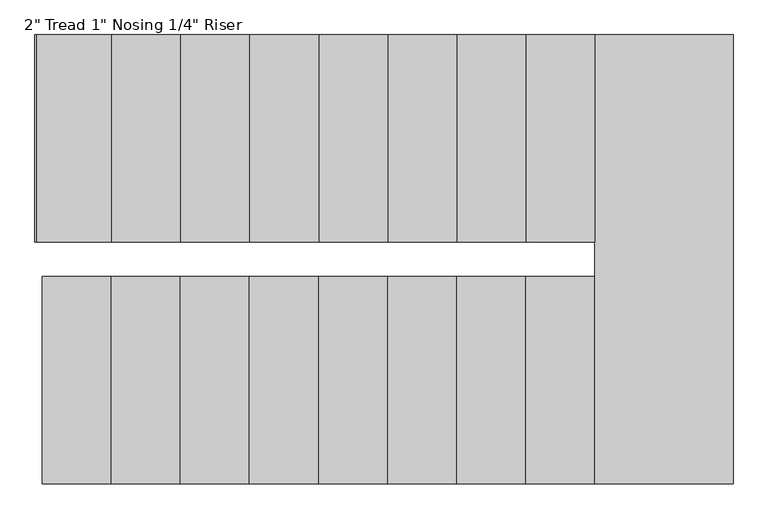
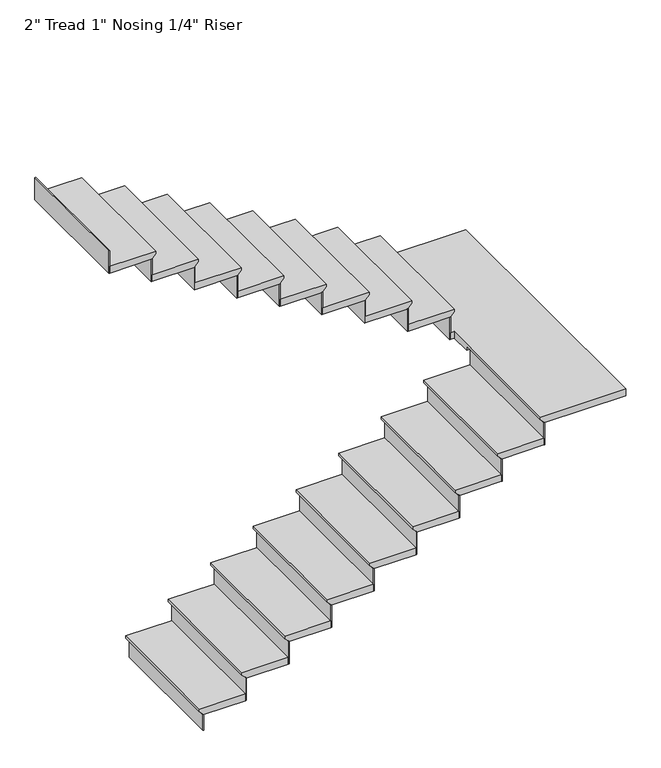
"""IFC4 building model written with IfcOpenShell, lengths in millimetres: stair flight geometry."""

from ifc_helpers import new_model, si_unit, origin, place, context, project, spatial, faceted_brep, source, transform, mapped, element, save


def stair_flight_21a7b5a9(model_context):
    return source(origin(), model_context, "Body", "Brep", [
        faceted_brep([(-1197.97188, -4816.50869, 3198.2833333), (-1197.97188, -4816.50869, 3217.3333333), (-1197.97188, -3902.10869, 3217.3333333), (-1197.97188, -3902.10869, 3198.2833333), (-1172.57188, -4816.50869, 3172.8833333), (-1172.57188, -3902.10869, 3172.8833333), (-867.77188, -4816.50869, 3217.3333333), (-867.77188, -3902.10869, 3217.3333333), (-1172.57188, -3902.10869, 3166.5333333), (-867.77188, -3902.10869, 3166.5333333), (-867.77188, -4816.50869, 3166.5333333), (-1172.57188, -4816.50869, 3166.5333333)], [[[0, 1, 2, 3]], [[4, 0, 3, 5]], [[2, 1, 6, 7]], [[8, 9, 10, 11]], [[2, 7, 9, 8, 5, 3]], [[8, 11, 4, 5]], [[6, 1, 0, 4, 11, 10]], [[7, 6, 10, 9]]]),
        faceted_brep([(-1172.57188, -4816.50869, 3166.5333333), (-1172.57188, -4816.50869, 3048.0), (-1166.22188, -4816.50869, 3048.0), (-1166.22188, -4816.50869, 3166.5333333), (-1172.57188, -3902.10869, 3166.5333333), (-1166.22188, -3902.10869, 3166.5333333), (-1166.22188, -3902.10869, 3048.0), (-1172.57188, -3902.10869, 3048.0)], [[[0, 1, 2, 3]], [[4, 5, 6, 7]], [[1, 0, 4, 7]], [[2, 1, 7, 6]], [[3, 2, 6, 5]], [[0, 3, 5, 4]]]),
        faceted_brep([(-867.77188, -4816.50869, 3335.8666667), (-867.77188, -4816.50869, 3166.5333333), (-861.42188, -4816.50869, 3166.5333333), (-861.42188, -4816.50869, 3335.8666667), (-867.77188, -3902.10869, 3335.8666667), (-861.42188, -3902.10869, 3335.8666667), (-861.42188, -3902.10869, 3166.5333333), (-867.77188, -3902.10869, 3166.5333333)], [[[0, 1, 2, 3]], [[4, 5, 6, 7]], [[1, 0, 4, 7]], [[2, 1, 7, 6]], [[3, 2, 6, 5]], [[0, 3, 5, 4]]]),
        faceted_brep([(-893.17188, -3902.10869, 3386.6666667), (-893.17188, -4816.50869, 3386.6666667), (-562.97188, -4816.50869, 3386.6666667), (-562.97188, -3902.10869, 3386.6666667), (-867.77188, -3902.10869, 3335.8666667), (-562.97188, -3902.10869, 3335.8666667), (-562.97188, -4816.50869, 3335.8666667), (-867.77188, -4816.50869, 3335.8666667), (-867.77188, -3902.10869, 3342.2166667), (-893.17188, -3902.10869, 3367.6166667), (-867.77188, -4816.50869, 3342.2166667), (-893.17188, -4816.50869, 3367.6166667)], [[[0, 1, 2, 3]], [[4, 5, 6, 7]], [[0, 3, 5, 4, 8, 9]], [[4, 7, 10, 8]], [[2, 1, 11, 10, 7, 6]], [[3, 2, 6, 5]], [[11, 1, 0, 9]], [[10, 11, 9, 8]]]),
        faceted_brep([(-562.97188, -4816.50869, 3505.2), (-562.97188, -4816.50869, 3335.8666667), (-556.62188, -4816.50869, 3335.8666667), (-556.62188, -4816.50869, 3505.2), (-562.97188, -3902.10869, 3505.2), (-556.62188, -3902.10869, 3505.2), (-556.62188, -3902.10869, 3335.8666667), (-562.97188, -3902.10869, 3335.8666667)], [[[0, 1, 2, 3]], [[4, 5, 6, 7]], [[1, 0, 4, 7]], [[2, 1, 7, 6]], [[3, 2, 6, 5]], [[0, 3, 5, 4]]]),
        faceted_brep([(-588.37188, -3902.10869, 3556.0), (-588.37188, -4816.50869, 3556.0), (-258.17188, -4816.50869, 3556.0), (-258.17188, -3902.10869, 3556.0), (-562.97188, -3902.10869, 3505.2), (-258.17188, -3902.10869, 3505.2), (-258.17188, -4816.50869, 3505.2), (-562.97188, -4816.50869, 3505.2), (-562.97188, -3902.10869, 3511.55), (-588.37188, -3902.10869, 3536.95), (-562.97188, -4816.50869, 3511.55), (-588.37188, -4816.50869, 3536.95)], [[[0, 1, 2, 3]], [[4, 5, 6, 7]], [[0, 3, 5, 4, 8, 9]], [[4, 7, 10, 8]], [[2, 1, 11, 10, 7, 6]], [[3, 2, 6, 5]], [[11, 1, 0, 9]], [[10, 11, 9, 8]]]),
        faceted_brep([(-258.17188, -4816.50869, 3674.5333333), (-258.17188, -4816.50869, 3505.2), (-251.82188, -4816.50869, 3505.2), (-251.82188, -4816.50869, 3674.5333333), (-258.17188, -3902.10869, 3674.5333333), (-251.82188, -3902.10869, 3674.5333333), (-251.82188, -3902.10869, 3505.2), (-258.17188, -3902.10869, 3505.2)], [[[0, 1, 2, 3]], [[4, 5, 6, 7]], [[1, 0, 4, 7]], [[2, 1, 7, 6]], [[3, 2, 6, 5]], [[0, 3, 5, 4]]]),
        faceted_brep([(-283.57188, -3902.10869, 3725.3333333), (-283.57188, -4816.50869, 3725.3333333), (46.62812, -4816.50869, 3725.3333333), (46.62812, -3902.10869, 3725.3333333), (-258.17188, -3902.10869, 3674.5333333), (46.62812, -3902.10869, 3674.5333333), (46.62812, -4816.50869, 3674.5333333), (-258.17188, -4816.50869, 3674.5333333), (-258.17188, -3902.10869, 3680.8833333), (-283.57188, -3902.10869, 3706.2833333), (-258.17188, -4816.50869, 3680.8833333), (-283.57188, -4816.50869, 3706.2833333)], [[[0, 1, 2, 3]], [[4, 5, 6, 7]], [[0, 3, 5, 4, 8, 9]], [[4, 7, 10, 8]], [[2, 1, 11, 10, 7, 6]], [[3, 2, 6, 5]], [[11, 1, 0, 9]], [[10, 11, 9, 8]]]),
        faceted_brep([(46.62812, -4816.50869, 3843.8666667), (46.62812, -4816.50869, 3674.5333333), (52.97812, -4816.50869, 3674.5333333), (52.97812, -4816.50869, 3843.8666667), (46.62812, -3902.10869, 3843.8666667), (52.97812, -3902.10869, 3843.8666667), (52.97812, -3902.10869, 3674.5333333), (46.62812, -3902.10869, 3674.5333333)], [[[0, 1, 2, 3]], [[4, 5, 6, 7]], [[1, 0, 4, 7]], [[2, 1, 7, 6]], [[3, 2, 6, 5]], [[0, 3, 5, 4]]]),
        faceted_brep([(21.22812, -3902.10869, 3894.6666667), (21.22812, -4816.50869, 3894.6666667), (351.42812, -4816.50869, 3894.6666667), (351.42812, -3902.10869, 3894.6666667), (46.62812, -3902.10869, 3843.8666667), (351.42812, -3902.10869, 3843.8666667), (351.42812, -4816.50869, 3843.8666667), (46.62812, -4816.50869, 3843.8666667), (46.62812, -3902.10869, 3850.2166667), (21.22812, -3902.10869, 3875.6166667), (46.62812, -4816.50869, 3850.2166667), (21.22812, -4816.50869, 3875.6166667)], [[[0, 1, 2, 3]], [[4, 5, 6, 7]], [[0, 3, 5, 4, 8, 9]], [[4, 7, 10, 8]], [[2, 1, 11, 10, 7, 6]], [[3, 2, 6, 5]], [[11, 1, 0, 9]], [[10, 11, 9, 8]]]),
        faceted_brep([(351.42812, -4816.50869, 4013.2), (351.42812, -4816.50869, 3843.8666667), (357.77812, -4816.50869, 3843.8666667), (357.77812, -4816.50869, 4013.2), (351.42812, -3902.10869, 4013.2), (357.77812, -3902.10869, 4013.2), (357.77812, -3902.10869, 3843.8666667), (351.42812, -3902.10869, 3843.8666667)], [[[0, 1, 2, 3]], [[4, 5, 6, 7]], [[1, 0, 4, 7]], [[2, 1, 7, 6]], [[3, 2, 6, 5]], [[0, 3, 5, 4]]]),
        faceted_brep([(326.02812, -3902.10869, 4064.0), (326.02812, -4816.50869, 4064.0), (656.22812, -4816.50869, 4064.0), (656.22812, -3902.10869, 4064.0), (351.42812, -3902.10869, 4013.2), (656.22812, -3902.10869, 4013.2), (656.22812, -4816.50869, 4013.2), (351.42812, -4816.50869, 4013.2), (351.42812, -3902.10869, 4019.55), (326.02812, -3902.10869, 4044.95), (351.42812, -4816.50869, 4019.55), (326.02812, -4816.50869, 4044.95)], [[[0, 1, 2, 3]], [[4, 5, 6, 7]], [[0, 3, 5, 4, 8, 9]], [[4, 7, 10, 8]], [[2, 1, 11, 10, 7, 6]], [[3, 2, 6, 5]], [[11, 1, 0, 9]], [[10, 11, 9, 8]]]),
        faceted_brep([(656.22812, -4816.50869, 4182.5333333), (656.22812, -4816.50869, 4013.2), (662.57812, -4816.50869, 4013.2), (662.57812, -4816.50869, 4182.5333333), (656.22812, -3902.10869, 4182.5333333), (662.57812, -3902.10869, 4182.5333333), (662.57812, -3902.10869, 4013.2), (656.22812, -3902.10869, 4013.2)], [[[0, 1, 2, 3]], [[4, 5, 6, 7]], [[1, 0, 4, 7]], [[2, 1, 7, 6]], [[3, 2, 6, 5]], [[0, 3, 5, 4]]]),
        faceted_brep([(630.82812, -3902.10869, 4233.3333333), (630.82812, -4816.50869, 4233.3333333), (961.02812, -4816.50869, 4233.3333333), (961.02812, -3902.10869, 4233.3333333), (656.22812, -3902.10869, 4182.5333333), (961.02812, -3902.10869, 4182.5333333), (961.02812, -4816.50869, 4182.5333333), (656.22812, -4816.50869, 4182.5333333), (656.22812, -3902.10869, 4188.8833333), (630.82812, -3902.10869, 4214.2833333), (656.22812, -4816.50869, 4188.8833333), (630.82812, -4816.50869, 4214.2833333)], [[[0, 1, 2, 3]], [[4, 5, 6, 7]], [[0, 3, 5, 4, 8, 9]], [[4, 7, 10, 8]], [[2, 1, 11, 10, 7, 6]], [[3, 2, 6, 5]], [[11, 1, 0, 9]], [[10, 11, 9, 8]]]),
        faceted_brep([(961.02812, -4816.50869, 4351.8666667), (961.02812, -4816.50869, 4182.5333333), (967.37812, -4816.50869, 4182.5333333), (967.37812, -4816.50869, 4351.8666667), (961.02812, -3902.10869, 4351.8666667), (967.37812, -3902.10869, 4351.8666667), (967.37812, -3902.10869, 4182.5333333), (961.02812, -3902.10869, 4182.5333333)], [[[0, 1, 2, 3]], [[4, 5, 6, 7]], [[1, 0, 4, 7]], [[2, 1, 7, 6]], [[3, 2, 6, 5]], [[0, 3, 5, 4]]]),
        faceted_brep([(935.62812, -3902.10869, 4402.6666667), (935.62812, -4816.50869, 4402.6666667), (1265.82812, -4816.50869, 4402.6666667), (1265.82812, -3902.10869, 4402.6666667), (961.02812, -3902.10869, 4351.8666667), (1265.82812, -3902.10869, 4351.8666667), (1265.82812, -4816.50869, 4351.8666667), (961.02812, -4816.50869, 4351.8666667), (961.02812, -3902.10869, 4358.2166667), (935.62812, -3902.10869, 4383.6166667), (961.02812, -4816.50869, 4358.2166667), (935.62812, -4816.50869, 4383.6166667)], [[[0, 1, 2, 3]], [[4, 5, 6, 7]], [[0, 3, 5, 4, 8, 9]], [[4, 7, 10, 8]], [[2, 1, 11, 10, 7, 6]], [[3, 2, 6, 5]], [[11, 1, 0, 9]], [[10, 11, 9, 8]]]),
        faceted_brep([(1265.82812, -4816.50869, 4521.2), (1265.82812, -4816.50869, 4351.8666667), (1272.17812, -4816.50869, 4351.8666667), (1272.17812, -4816.50869, 4521.2), (1265.82812, -3902.10869, 4521.2), (1272.17812, -3902.10869, 4521.2), (1272.17812, -3902.10869, 4351.8666667), (1265.82812, -3902.10869, 4351.8666667)], [[[0, 1, 2, 3]], [[4, 5, 6, 7]], [[1, 0, 4, 7]], [[2, 1, 7, 6]], [[3, 2, 6, 5]], [[0, 3, 5, 4]]]),
        faceted_brep([(1215.02812, -3749.70869, 4572.0), (1240.42812, -3749.70869, 4572.0), (1240.42812, -4816.50869, 4572.0), (1850.02812, -4816.50869, 4572.0), (1850.02812, -2835.30869, 4572.0), (1215.02812, -2835.30869, 4572.0), (1240.42812, -3749.70869, 4521.2), (1215.02812, -3749.70869, 4521.2), (1215.02812, -2835.30869, 4521.2), (1850.02812, -2835.30869, 4521.2), (1850.02812, -4816.50869, 4521.2), (1265.82812, -4816.50869, 4521.2), (1265.82812, -3902.10869, 4521.2), (1240.42812, -3902.10869, 4521.2), (1240.42812, -3902.10869, 4552.95), (1240.42812, -4816.50869, 4552.95), (1265.82812, -3902.10869, 4527.55), (1265.82812, -4816.50869, 4527.55)], [[[0, 1, 2, 3, 4, 5]], [[6, 7, 8, 9, 10, 11, 12, 13]], [[1, 0, 7, 6]], [[2, 1, 6, 13, 14, 15]], [[13, 12, 16, 14]], [[12, 11, 17, 16]], [[3, 2, 15, 17, 11, 10]], [[4, 3, 10, 9]], [[5, 4, 9, 8]], [[0, 5, 8, 7]], [[17, 15, 14, 16]]]),
        faceted_brep([(1215.02812, -2835.30869, 4690.5333333), (1215.02812, -2835.30869, 4521.2), (1208.67812, -2835.30869, 4521.2), (1208.67812, -2835.30869, 4690.5333333), (1215.02812, -3749.70869, 4690.5333333), (1208.67812, -3749.70869, 4690.5333333), (1208.67812, -3749.70869, 4521.2), (1215.02812, -3749.70869, 4521.2)], [[[0, 1, 2, 3]], [[4, 5, 6, 7]], [[1, 0, 4, 7]], [[2, 1, 7, 6]], [[3, 2, 6, 5]], [[0, 3, 5, 4]]]),
        faceted_brep([(1240.42812, -3749.70869, 4741.3333333), (1240.42812, -2835.30869, 4741.3333333), (910.22812, -2835.30869, 4741.3333333), (910.22812, -3749.70869, 4741.3333333), (1215.02812, -3749.70869, 4690.5333333), (910.22812, -3749.70869, 4690.5333333), (910.22812, -2835.30869, 4690.5333333), (1215.02812, -2835.30869, 4690.5333333), (1215.02812, -3749.70869, 4696.8833333), (1240.42812, -3749.70869, 4722.2833333), (1215.02812, -2835.30869, 4696.8833333), (1240.42812, -2835.30869, 4722.2833333)], [[[0, 1, 2, 3]], [[4, 5, 6, 7]], [[0, 3, 5, 4, 8, 9]], [[4, 7, 10, 8]], [[2, 1, 11, 10, 7, 6]], [[3, 2, 6, 5]], [[11, 1, 0, 9]], [[10, 11, 9, 8]]]),
        faceted_brep([(910.22812, -2835.30869, 4859.8666667), (910.22812, -2835.30869, 4690.5333333), (903.87812, -2835.30869, 4690.5333333), (903.87812, -2835.30869, 4859.8666667), (910.22812, -3749.70869, 4859.8666667), (903.87812, -3749.70869, 4859.8666667), (903.87812, -3749.70869, 4690.5333333), (910.22812, -3749.70869, 4690.5333333)], [[[0, 1, 2, 3]], [[4, 5, 6, 7]], [[1, 0, 4, 7]], [[2, 1, 7, 6]], [[3, 2, 6, 5]], [[0, 3, 5, 4]]]),
        faceted_brep([(935.62812, -3749.70869, 4910.6666667), (935.62812, -2835.30869, 4910.6666667), (605.42812, -2835.30869, 4910.6666667), (605.42812, -3749.70869, 4910.6666667), (910.22812, -3749.70869, 4859.8666667), (605.42812, -3749.70869, 4859.8666667), (605.42812, -2835.30869, 4859.8666667), (910.22812, -2835.30869, 4859.8666667), (910.22812, -3749.70869, 4866.2166667), (935.62812, -3749.70869, 4891.6166667), (910.22812, -2835.30869, 4866.2166667), (935.62812, -2835.30869, 4891.6166667)], [[[0, 1, 2, 3]], [[4, 5, 6, 7]], [[0, 3, 5, 4, 8, 9]], [[4, 7, 10, 8]], [[2, 1, 11, 10, 7, 6]], [[3, 2, 6, 5]], [[11, 1, 0, 9]], [[10, 11, 9, 8]]]),
        faceted_brep([(605.42812, -2835.30869, 5029.2), (605.42812, -2835.30869, 4859.8666667), (599.07812, -2835.30869, 4859.8666667), (599.07812, -2835.30869, 5029.2), (605.42812, -3749.70869, 5029.2), (599.07812, -3749.70869, 5029.2), (599.07812, -3749.70869, 4859.8666667), (605.42812, -3749.70869, 4859.8666667)], [[[0, 1, 2, 3]], [[4, 5, 6, 7]], [[1, 0, 4, 7]], [[2, 1, 7, 6]], [[3, 2, 6, 5]], [[0, 3, 5, 4]]]),
        faceted_brep([(630.82812, -3749.70869, 5080.0), (630.82812, -2835.30869, 5080.0), (300.62812, -2835.30869, 5080.0), (300.62812, -3749.70869, 5080.0), (605.42812, -3749.70869, 5029.2), (300.62812, -3749.70869, 5029.2), (300.62812, -2835.30869, 5029.2), (605.42812, -2835.30869, 5029.2), (605.42812, -3749.70869, 5035.55), (630.82812, -3749.70869, 5060.95), (605.42812, -2835.30869, 5035.55), (630.82812, -2835.30869, 5060.95)], [[[0, 1, 2, 3]], [[4, 5, 6, 7]], [[0, 3, 5, 4, 8, 9]], [[4, 7, 10, 8]], [[2, 1, 11, 10, 7, 6]], [[3, 2, 6, 5]], [[11, 1, 0, 9]], [[10, 11, 9, 8]]]),
        faceted_brep([(300.62812, -2835.30869, 5198.5333333), (300.62812, -2835.30869, 5029.2), (294.27812, -2835.30869, 5029.2), (294.27812, -2835.30869, 5198.5333333), (300.62812, -3749.70869, 5198.5333333), (294.27812, -3749.70869, 5198.5333333), (294.27812, -3749.70869, 5029.2), (300.62812, -3749.70869, 5029.2)], [[[0, 1, 2, 3]], [[4, 5, 6, 7]], [[1, 0, 4, 7]], [[2, 1, 7, 6]], [[3, 2, 6, 5]], [[0, 3, 5, 4]]]),
        faceted_brep([(326.02812, -3749.70869, 5249.3333333), (326.02812, -2835.30869, 5249.3333333), (-4.17188, -2835.30869, 5249.3333333), (-4.17188, -3749.70869, 5249.3333333), (300.62812, -3749.70869, 5198.5333333), (-4.17188, -3749.70869, 5198.5333333), (-4.17188, -2835.30869, 5198.5333333), (300.62812, -2835.30869, 5198.5333333), (300.62812, -3749.70869, 5204.8833333), (326.02812, -3749.70869, 5230.2833333), (300.62812, -2835.30869, 5204.8833333), (326.02812, -2835.30869, 5230.2833333)], [[[0, 1, 2, 3]], [[4, 5, 6, 7]], [[0, 3, 5, 4, 8, 9]], [[4, 7, 10, 8]], [[2, 1, 11, 10, 7, 6]], [[3, 2, 6, 5]], [[11, 1, 0, 9]], [[10, 11, 9, 8]]]),
        faceted_brep([(-4.17188, -2835.30869, 5367.8666667), (-4.17188, -2835.30869, 5198.5333333), (-10.52188, -2835.30869, 5198.5333333), (-10.52188, -2835.30869, 5367.8666667), (-4.17188, -3749.70869, 5367.8666667), (-10.52188, -3749.70869, 5367.8666667), (-10.52188, -3749.70869, 5198.5333333), (-4.17188, -3749.70869, 5198.5333333)], [[[0, 1, 2, 3]], [[4, 5, 6, 7]], [[1, 0, 4, 7]], [[2, 1, 7, 6]], [[3, 2, 6, 5]], [[0, 3, 5, 4]]]),
        faceted_brep([(21.22812, -3749.70869, 5418.6666667), (21.22812, -2835.30869, 5418.6666667), (-308.97188, -2835.30869, 5418.6666667), (-308.97188, -3749.70869, 5418.6666667), (-4.17188, -3749.70869, 5367.8666667), (-308.97188, -3749.70869, 5367.8666667), (-308.97188, -2835.30869, 5367.8666667), (-4.17188, -2835.30869, 5367.8666667), (-4.17188, -3749.70869, 5374.2166667), (21.22812, -3749.70869, 5399.6166667), (-4.17188, -2835.30869, 5374.2166667), (21.22812, -2835.30869, 5399.6166667)], [[[0, 1, 2, 3]], [[4, 5, 6, 7]], [[0, 3, 5, 4, 8, 9]], [[4, 7, 10, 8]], [[2, 1, 11, 10, 7, 6]], [[3, 2, 6, 5]], [[11, 1, 0, 9]], [[10, 11, 9, 8]]]),
        faceted_brep([(-308.97188, -2835.30869, 5537.2), (-308.97188, -2835.30869, 5367.8666667), (-315.32188, -2835.30869, 5367.8666667), (-315.32188, -2835.30869, 5537.2), (-308.97188, -3749.70869, 5537.2), (-315.32188, -3749.70869, 5537.2), (-315.32188, -3749.70869, 5367.8666667), (-308.97188, -3749.70869, 5367.8666667)], [[[0, 1, 2, 3]], [[4, 5, 6, 7]], [[1, 0, 4, 7]], [[2, 1, 7, 6]], [[3, 2, 6, 5]], [[0, 3, 5, 4]]]),
        faceted_brep([(-283.57188, -3749.70869, 5588.0), (-283.57188, -2835.30869, 5588.0), (-613.77188, -2835.30869, 5588.0), (-613.77188, -3749.70869, 5588.0), (-308.97188, -3749.70869, 5537.2), (-613.77188, -3749.70869, 5537.2), (-613.77188, -2835.30869, 5537.2), (-308.97188, -2835.30869, 5537.2), (-308.97188, -3749.70869, 5543.55), (-283.57188, -3749.70869, 5568.95), (-308.97188, -2835.30869, 5543.55), (-283.57188, -2835.30869, 5568.95)], [[[0, 1, 2, 3]], [[4, 5, 6, 7]], [[0, 3, 5, 4, 8, 9]], [[4, 7, 10, 8]], [[2, 1, 11, 10, 7, 6]], [[3, 2, 6, 5]], [[11, 1, 0, 9]], [[10, 11, 9, 8]]]),
        faceted_brep([(-613.77188, -2835.30869, 5706.5333333), (-613.77188, -2835.30869, 5537.2), (-620.12188, -2835.30869, 5537.2), (-620.12188, -2835.30869, 5706.5333333), (-613.77188, -3749.70869, 5706.5333333), (-620.12188, -3749.70869, 5706.5333333), (-620.12188, -3749.70869, 5537.2), (-613.77188, -3749.70869, 5537.2)], [[[0, 1, 2, 3]], [[4, 5, 6, 7]], [[1, 0, 4, 7]], [[2, 1, 7, 6]], [[3, 2, 6, 5]], [[0, 3, 5, 4]]]),
        faceted_brep([(-588.37188, -3749.70869, 5757.3333333), (-588.37188, -2835.30869, 5757.3333333), (-918.57188, -2835.30869, 5757.3333333), (-918.57188, -3749.70869, 5757.3333333), (-613.77188, -3749.70869, 5706.5333333), (-918.57188, -3749.70869, 5706.5333333), (-918.57188, -2835.30869, 5706.5333333), (-613.77188, -2835.30869, 5706.5333333), (-613.77188, -3749.70869, 5712.8833333), (-588.37188, -3749.70869, 5738.2833333), (-613.77188, -2835.30869, 5712.8833333), (-588.37188, -2835.30869, 5738.2833333)], [[[0, 1, 2, 3]], [[4, 5, 6, 7]], [[0, 3, 5, 4, 8, 9]], [[4, 7, 10, 8]], [[2, 1, 11, 10, 7, 6]], [[3, 2, 6, 5]], [[11, 1, 0, 9]], [[10, 11, 9, 8]]]),
        faceted_brep([(-918.57188, -2835.30869, 5875.8666667), (-918.57188, -2835.30869, 5706.5333333), (-924.92188, -2835.30869, 5706.5333333), (-924.92188, -2835.30869, 5875.8666667), (-918.57188, -3749.70869, 5875.8666667), (-924.92188, -3749.70869, 5875.8666667), (-924.92188, -3749.70869, 5706.5333333), (-918.57188, -3749.70869, 5706.5333333)], [[[0, 1, 2, 3]], [[4, 5, 6, 7]], [[1, 0, 4, 7]], [[2, 1, 7, 6]], [[3, 2, 6, 5]], [[0, 3, 5, 4]]]),
        faceted_brep([(-1223.37188, -2835.30869, 6045.2), (-1223.37188, -2835.30869, 5875.8666667), (-1229.72188, -2835.30869, 5875.8666667), (-1229.72188, -2835.30869, 6045.2), (-1223.37188, -3749.70869, 6045.2), (-1229.72188, -3749.70869, 6045.2), (-1229.72188, -3749.70869, 5875.8666667), (-1223.37188, -3749.70869, 5875.8666667)], [[[0, 1, 2, 3]], [[4, 5, 6, 7]], [[1, 0, 4, 7]], [[2, 1, 7, 6]], [[3, 2, 6, 5]], [[0, 3, 5, 4]]]),
        faceted_brep([(-893.17188, -3749.70869, 5926.6666667), (-893.17188, -2835.30869, 5926.6666667), (-1223.37188, -2835.30869, 5926.6666667), (-1223.37188, -3749.70869, 5926.6666667), (-918.57188, -3749.70869, 5875.8666667), (-1223.37188, -3749.70869, 5875.8666667), (-1223.37188, -2835.30869, 5875.8666667), (-918.57188, -2835.30869, 5875.8666667), (-918.57188, -3749.70869, 5882.2166667), (-893.17188, -3749.70869, 5907.6166667), (-918.57188, -2835.30869, 5882.2166667), (-893.17188, -2835.30869, 5907.6166667)], [[[0, 1, 2, 3]], [[4, 5, 6, 7]], [[0, 3, 5, 4, 8, 9]], [[4, 7, 10, 8]], [[2, 1, 11, 10, 7, 6]], [[3, 2, 6, 5]], [[11, 1, 0, 9]], [[10, 11, 9, 8]]]),
    ])


if __name__ == "__main__":
    model = new_model("IFC4")
    model_context = context("Model", 3, world=origin())
    ifc_project = project(units=[si_unit("LENGTHUNIT", "METRE", prefix="MILLI")], contexts=[model_context])
    site = spatial("IfcSite", under=ifc_project)
    building = spatial("IfcBuilding", under=site)
    placement = place(None, origin())
    stair_flight_shape = stair_flight_21a7b5a9(model_context)
    element("IfcStairFlight", 1, ObjectType="2\" Tread 1\" Nosing 1/4\" Riser", at=placement, inside=building, context=model_context, shape_type="MappedRepresentation", body=[
        mapped(stair_flight_shape, transform((0.0, 0.0, 0.0), x_axis=(1.0, 0.0, 0.0), y_axis=(0.0, 1.0, 0.0), z_axis=(0.0, 0.0, 1.0))),
    ])
    save(model, "model.ifc")
